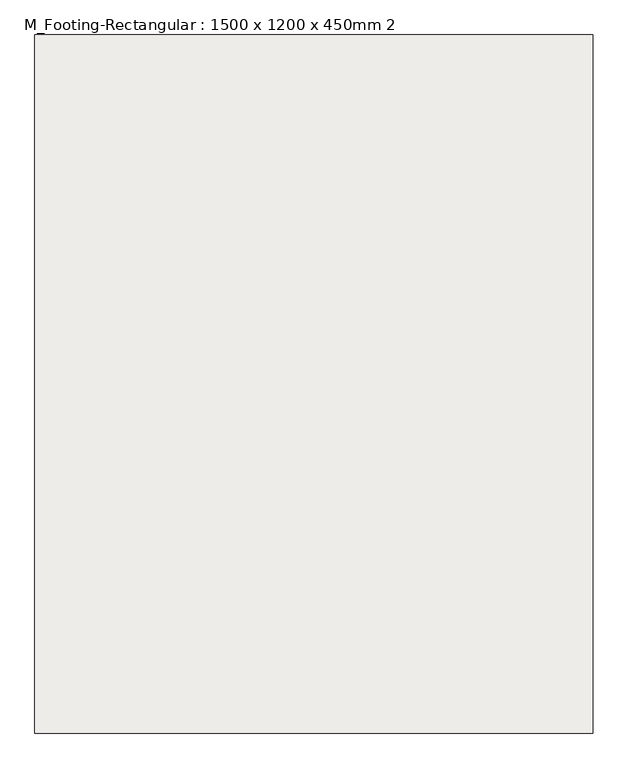
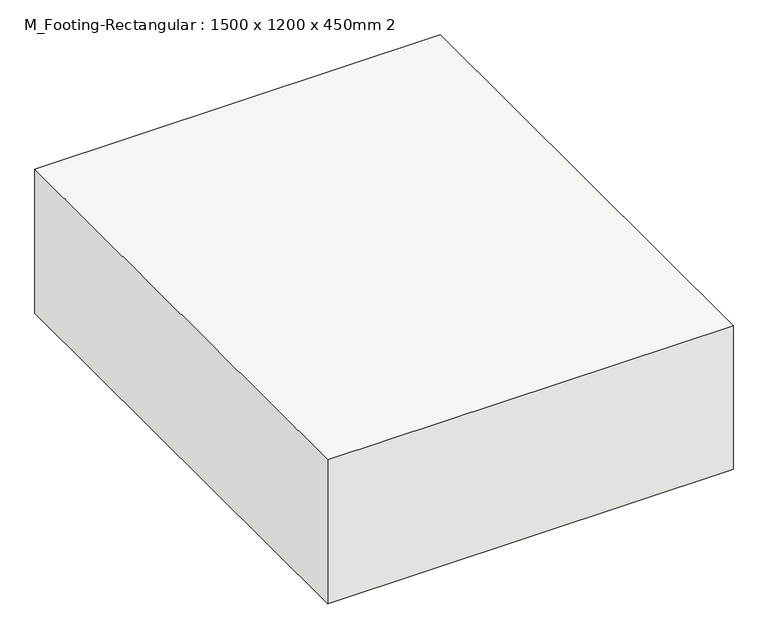
"""IFC4 building model written with IfcOpenShell, lengths in millimetres: slab geometry, M_Footing-Rectangular : 1500 x 1200 x 450mm 2."""

from ifc_helpers import new_model, si_unit, frame, origin, place, context, project, spatial, polyline, outline, extrude, source, transform, mapped, element, save


def m_footing_rectangular_1500_x_1200_x_450mm_2_af0c1bbe(model_context):
    return source(origin(), model_context, "Body", "SweptSolid", [
        extrude(outline(polyline([(600.0, 750.0), (600.0, -750.0), (-600.0, -750.0), (-600.0, 750.0), (600.0, 750.0)])), frame((0.0, 0.0, -450.0), z_axis=(0.0, 0.0, 1.0), x_axis=(1.0, 0.0, 0.0)), (0.0, 0.0, 1.0), 450.0),
    ])


if __name__ == "__main__":
    model = new_model("IFC4")
    model_context = context("Model", 3, world=origin())
    ifc_project = project(units=[si_unit("LENGTHUNIT", "METRE", prefix="MILLI")], contexts=[model_context])
    site = spatial("IfcSite", under=ifc_project)
    building = spatial("IfcBuilding", under=site)
    placement = place(None, origin())
    m_footing_rectangular_1500_x_1200_x_450mm_2_shape = m_footing_rectangular_1500_x_1200_x_450mm_2_af0c1bbe(model_context)
    element("IfcSlab", 1, ObjectType="M_Footing-Rectangular : 1500 x 1200 x 450mm 2", at=placement, inside=building, context=model_context, shape_type="MappedRepresentation", body=[
        mapped(m_footing_rectangular_1500_x_1200_x_450mm_2_shape, transform((0.0, 0.0, 0.0), x_axis=(1.0, 0.0, 0.0), y_axis=(0.0, 1.0, 0.0), z_axis=(0.0, 0.0, 1.0))),
    ])
    save(model, "model.ifc")

# Revit data of these elements
# Type "M_Footing-Rectangular : 1500 x 1200 x 450mm 2"
#   Width = 3' - 11.24409"
#   Length = 4' - 11.05512"
#   Foundation Thickness = 1' - 5.71654"
#   Structural Material [instance default] = Concrete, Cast-in-Place gray
#   Assembly Code = ""
# Element 1 (IfcSlab, "M_Footing-Rectangular : 1500 x 1200 x 450mm 2")
#   Materials on its faces: "Concrete, Cast-in-Place gray"
# Materials
#   "Concrete, Cast-in-Place gray": class "Concrete", colour RGB 192 192 192, transparency 0, Description = "Cast-in-place concrete", Cost = 0
